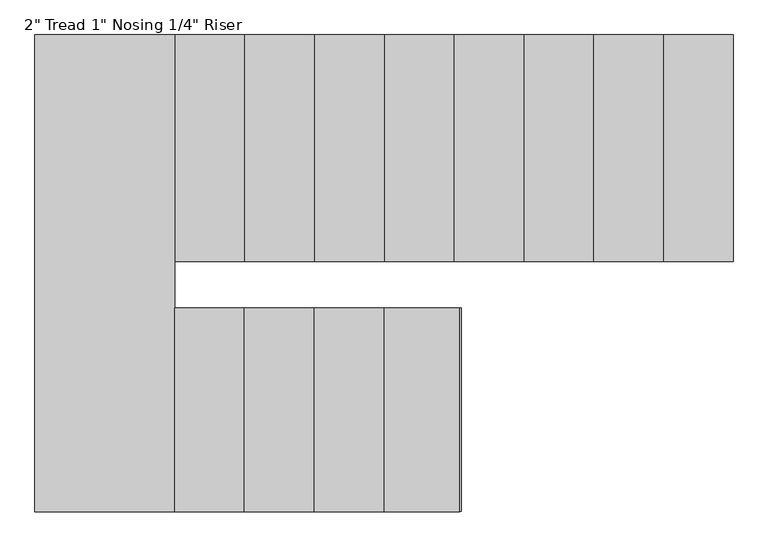
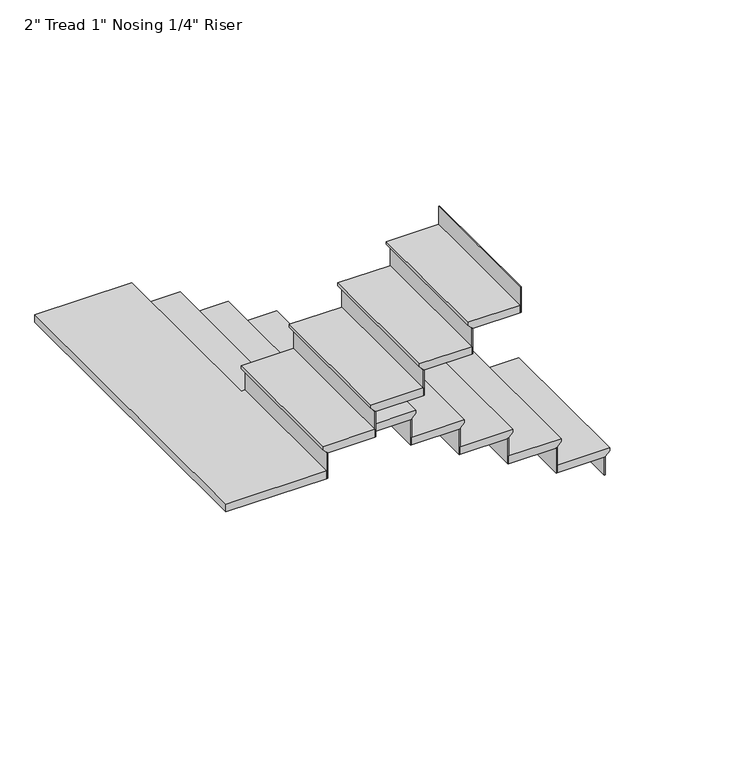
"""IFC4 building model written with IfcOpenShell, lengths in millimetres: stair flight geometry."""

from ifc_helpers import new_model, si_unit, origin, place, context, project, spatial, faceted_brep, source, transform, mapped, element, save


def stair_flight_da212e09(model_context):
    return source(origin(), model_context, "Body", "Brep", [
        faceted_brep([(-569.5630704, 657.3457979, 6398.6833333), (-569.5630704, 657.3457979, 6417.7333333), (-569.5630704, -333.2542021, 6417.7333333), (-569.5630704, -333.2542021, 6398.6833333), (-594.9630704, 657.3457979, 6373.2833333), (-594.9630704, -333.2542021, 6373.2833333), (-899.7630704, 657.3457979, 6417.7333333), (-899.7630704, -333.2542021, 6417.7333333), (-594.9630704, -333.2542021, 6366.9333333), (-899.7630704, -333.2542021, 6366.9333333), (-899.7630704, 657.3457979, 6366.9333333), (-594.9630704, 657.3457979, 6366.9333333)], [[[0, 1, 2, 3]], [[4, 0, 3, 5]], [[2, 1, 6, 7]], [[8, 9, 10, 11]], [[2, 7, 9, 8, 5, 3]], [[8, 11, 4, 5]], [[6, 1, 0, 4, 11, 10]], [[7, 6, 10, 9]]]),
        faceted_brep([(-594.9630704, 657.3457979, 6366.9333333), (-594.9630704, 657.3457979, 6248.4), (-601.3130704, 657.3457979, 6248.4), (-601.3130704, 657.3457979, 6366.9333333), (-594.9630704, -333.2542021, 6366.9333333), (-601.3130704, -333.2542021, 6366.9333333), (-601.3130704, -333.2542021, 6248.4), (-594.9630704, -333.2542021, 6248.4)], [[[0, 1, 2, 3]], [[4, 5, 6, 7]], [[1, 0, 4, 7]], [[2, 1, 7, 6]], [[3, 2, 6, 5]], [[0, 3, 5, 4]]]),
        faceted_brep([(-899.7630704, 657.3457979, 6536.2666667), (-899.7630704, 657.3457979, 6366.9333333), (-906.1130704, 657.3457979, 6366.9333333), (-906.1130704, 657.3457979, 6536.2666667), (-899.7630704, -333.2542021, 6536.2666667), (-906.1130704, -333.2542021, 6536.2666667), (-906.1130704, -333.2542021, 6366.9333333), (-899.7630704, -333.2542021, 6366.9333333)], [[[0, 1, 2, 3]], [[4, 5, 6, 7]], [[1, 0, 4, 7]], [[2, 1, 7, 6]], [[3, 2, 6, 5]], [[0, 3, 5, 4]]]),
        faceted_brep([(-874.3630704, -333.2542021, 6587.0666667), (-874.3630704, 657.3457979, 6587.0666667), (-1204.5630704, 657.3457979, 6587.0666667), (-1204.5630704, -333.2542021, 6587.0666667), (-899.7630704, -333.2542021, 6536.2666667), (-1204.5630704, -333.2542021, 6536.2666667), (-1204.5630704, 657.3457979, 6536.2666667), (-899.7630704, 657.3457979, 6536.2666667), (-899.7630704, -333.2542021, 6542.6166667), (-874.3630704, -333.2542021, 6568.0166667), (-899.7630704, 657.3457979, 6542.6166667), (-874.3630704, 657.3457979, 6568.0166667)], [[[0, 1, 2, 3]], [[4, 5, 6, 7]], [[0, 3, 5, 4, 8, 9]], [[4, 7, 10, 8]], [[2, 1, 11, 10, 7, 6]], [[3, 2, 6, 5]], [[11, 1, 0, 9]], [[10, 11, 9, 8]]]),
        faceted_brep([(-1204.5630704, 657.3457979, 6705.6), (-1204.5630704, 657.3457979, 6536.2666667), (-1210.9130704, 657.3457979, 6536.2666667), (-1210.9130704, 657.3457979, 6705.6), (-1204.5630704, -333.2542021, 6705.6), (-1210.9130704, -333.2542021, 6705.6), (-1210.9130704, -333.2542021, 6536.2666667), (-1204.5630704, -333.2542021, 6536.2666667)], [[[0, 1, 2, 3]], [[4, 5, 6, 7]], [[1, 0, 4, 7]], [[2, 1, 7, 6]], [[3, 2, 6, 5]], [[0, 3, 5, 4]]]),
        faceted_brep([(-1179.1630704, -333.2542021, 6756.4), (-1179.1630704, 657.3457979, 6756.4), (-1509.3630704, 657.3457979, 6756.4), (-1509.3630704, -333.2542021, 6756.4), (-1204.5630704, -333.2542021, 6705.6), (-1509.3630704, -333.2542021, 6705.6), (-1509.3630704, 657.3457979, 6705.6), (-1204.5630704, 657.3457979, 6705.6), (-1204.5630704, -333.2542021, 6711.95), (-1179.1630704, -333.2542021, 6737.35), (-1204.5630704, 657.3457979, 6711.95), (-1179.1630704, 657.3457979, 6737.35)], [[[0, 1, 2, 3]], [[4, 5, 6, 7]], [[0, 3, 5, 4, 8, 9]], [[4, 7, 10, 8]], [[2, 1, 11, 10, 7, 6]], [[3, 2, 6, 5]], [[11, 1, 0, 9]], [[10, 11, 9, 8]]]),
        faceted_brep([(-1509.3630704, 657.3457979, 6874.9333333), (-1509.3630704, 657.3457979, 6705.6), (-1515.7130704, 657.3457979, 6705.6), (-1515.7130704, 657.3457979, 6874.9333333), (-1509.3630704, -333.2542021, 6874.9333333), (-1515.7130704, -333.2542021, 6874.9333333), (-1515.7130704, -333.2542021, 6705.6), (-1509.3630704, -333.2542021, 6705.6)], [[[0, 1, 2, 3]], [[4, 5, 6, 7]], [[1, 0, 4, 7]], [[2, 1, 7, 6]], [[3, 2, 6, 5]], [[0, 3, 5, 4]]]),
        faceted_brep([(-1483.9630704, -333.2542021, 6925.7333333), (-1483.9630704, 657.3457979, 6925.7333333), (-1814.1630704, 657.3457979, 6925.7333333), (-1814.1630704, -333.2542021, 6925.7333333), (-1509.3630704, -333.2542021, 6874.9333333), (-1814.1630704, -333.2542021, 6874.9333333), (-1814.1630704, 657.3457979, 6874.9333333), (-1509.3630704, 657.3457979, 6874.9333333), (-1509.3630704, -333.2542021, 6881.2833333), (-1483.9630704, -333.2542021, 6906.6833333), (-1509.3630704, 657.3457979, 6881.2833333), (-1483.9630704, 657.3457979, 6906.6833333)], [[[0, 1, 2, 3]], [[4, 5, 6, 7]], [[0, 3, 5, 4, 8, 9]], [[4, 7, 10, 8]], [[2, 1, 11, 10, 7, 6]], [[3, 2, 6, 5]], [[11, 1, 0, 9]], [[10, 11, 9, 8]]]),
        faceted_brep([(-1814.1630704, 657.3457979, 7044.2666667), (-1814.1630704, 657.3457979, 6874.9333333), (-1820.5130704, 657.3457979, 6874.9333333), (-1820.5130704, 657.3457979, 7044.2666667), (-1814.1630704, -333.2542021, 7044.2666667), (-1820.5130704, -333.2542021, 7044.2666667), (-1820.5130704, -333.2542021, 6874.9333333), (-1814.1630704, -333.2542021, 6874.9333333)], [[[0, 1, 2, 3]], [[4, 5, 6, 7]], [[1, 0, 4, 7]], [[2, 1, 7, 6]], [[3, 2, 6, 5]], [[0, 3, 5, 4]]]),
        faceted_brep([(-1788.7630704, -333.2542021, 7095.0666667), (-1788.7630704, 657.3457979, 7095.0666667), (-2118.9630704, 657.3457979, 7095.0666667), (-2118.9630704, -333.2542021, 7095.0666667), (-1814.1630704, -333.2542021, 7044.2666667), (-2118.9630704, -333.2542021, 7044.2666667), (-2118.9630704, 657.3457979, 7044.2666667), (-1814.1630704, 657.3457979, 7044.2666667), (-1814.1630704, -333.2542021, 7050.6166667), (-1788.7630704, -333.2542021, 7076.0166667), (-1814.1630704, 657.3457979, 7050.6166667), (-1788.7630704, 657.3457979, 7076.0166667)], [[[0, 1, 2, 3]], [[4, 5, 6, 7]], [[0, 3, 5, 4, 8, 9]], [[4, 7, 10, 8]], [[2, 1, 11, 10, 7, 6]], [[3, 2, 6, 5]], [[11, 1, 0, 9]], [[10, 11, 9, 8]]]),
        faceted_brep([(-2118.9630704, 657.3457979, 7213.6), (-2118.9630704, 657.3457979, 7044.2666667), (-2125.3130704, 657.3457979, 7044.2666667), (-2125.3130704, 657.3457979, 7213.6), (-2118.9630704, -333.2542021, 7213.6), (-2125.3130704, -333.2542021, 7213.6), (-2125.3130704, -333.2542021, 7044.2666667), (-2118.9630704, -333.2542021, 7044.2666667)], [[[0, 1, 2, 3]], [[4, 5, 6, 7]], [[1, 0, 4, 7]], [[2, 1, 7, 6]], [[3, 2, 6, 5]], [[0, 3, 5, 4]]]),
        faceted_brep([(-2093.5630704, -333.2542021, 7264.4), (-2093.5630704, 657.3457979, 7264.4), (-2423.7630704, 657.3457979, 7264.4), (-2423.7630704, -333.2542021, 7264.4), (-2118.9630704, -333.2542021, 7213.6), (-2423.7630704, -333.2542021, 7213.6), (-2423.7630704, 657.3457979, 7213.6), (-2118.9630704, 657.3457979, 7213.6), (-2118.9630704, -333.2542021, 7219.95), (-2093.5630704, -333.2542021, 7245.35), (-2118.9630704, 657.3457979, 7219.95), (-2093.5630704, 657.3457979, 7245.35)], [[[0, 1, 2, 3]], [[4, 5, 6, 7]], [[0, 3, 5, 4, 8, 9]], [[4, 7, 10, 8]], [[2, 1, 11, 10, 7, 6]], [[3, 2, 6, 5]], [[11, 1, 0, 9]], [[10, 11, 9, 8]]]),
        faceted_brep([(-2423.7630704, 657.3457979, 7382.9333333), (-2423.7630704, 657.3457979, 7213.6), (-2430.1130704, 657.3457979, 7213.6), (-2430.1130704, 657.3457979, 7382.9333333), (-2423.7630704, -333.2542021, 7382.9333333), (-2430.1130704, -333.2542021, 7382.9333333), (-2430.1130704, -333.2542021, 7213.6), (-2423.7630704, -333.2542021, 7213.6)], [[[0, 1, 2, 3]], [[4, 5, 6, 7]], [[1, 0, 4, 7]], [[2, 1, 7, 6]], [[3, 2, 6, 5]], [[0, 3, 5, 4]]]),
        faceted_brep([(-2398.3630704, -333.2542021, 7433.7333333), (-2398.3630704, 657.3457979, 7433.7333333), (-2728.5630704, 657.3457979, 7433.7333333), (-2728.5630704, -333.2542021, 7433.7333333), (-2423.7630704, -333.2542021, 7382.9333333), (-2728.5630704, -333.2542021, 7382.9333333), (-2728.5630704, 657.3457979, 7382.9333333), (-2423.7630704, 657.3457979, 7382.9333333), (-2423.7630704, -333.2542021, 7389.2833333), (-2398.3630704, -333.2542021, 7414.6833333), (-2423.7630704, 657.3457979, 7389.2833333), (-2398.3630704, 657.3457979, 7414.6833333)], [[[0, 1, 2, 3]], [[4, 5, 6, 7]], [[0, 3, 5, 4, 8, 9]], [[4, 7, 10, 8]], [[2, 1, 11, 10, 7, 6]], [[3, 2, 6, 5]], [[11, 1, 0, 9]], [[10, 11, 9, 8]]]),
        faceted_brep([(-2728.5630704, 657.3457979, 7552.2666667), (-2728.5630704, 657.3457979, 7382.9333333), (-2734.9130704, 657.3457979, 7382.9333333), (-2734.9130704, 657.3457979, 7552.2666667), (-2728.5630704, -333.2542021, 7552.2666667), (-2734.9130704, -333.2542021, 7552.2666667), (-2734.9130704, -333.2542021, 7382.9333333), (-2728.5630704, -333.2542021, 7382.9333333)], [[[0, 1, 2, 3]], [[4, 5, 6, 7]], [[1, 0, 4, 7]], [[2, 1, 7, 6]], [[3, 2, 6, 5]], [[0, 3, 5, 4]]]),
        faceted_brep([(-2703.1630704, -333.2542021, 7603.0666667), (-2703.1630704, 657.3457979, 7603.0666667), (-3033.3630704, 657.3457979, 7603.0666667), (-3033.3630704, -333.2542021, 7603.0666667), (-2728.5630704, -333.2542021, 7552.2666667), (-3033.3630704, -333.2542021, 7552.2666667), (-3033.3630704, 657.3457979, 7552.2666667), (-2728.5630704, 657.3457979, 7552.2666667), (-2728.5630704, -333.2542021, 7558.6166667), (-2703.1630704, -333.2542021, 7584.0166667), (-2728.5630704, 657.3457979, 7558.6166667), (-2703.1630704, 657.3457979, 7584.0166667)], [[[0, 1, 2, 3]], [[4, 5, 6, 7]], [[0, 3, 5, 4, 8, 9]], [[4, 7, 10, 8]], [[2, 1, 11, 10, 7, 6]], [[3, 2, 6, 5]], [[11, 1, 0, 9]], [[10, 11, 9, 8]]]),
        faceted_brep([(-3033.3630704, 657.3457979, 7721.6), (-3033.3630704, 657.3457979, 7552.2666667), (-3039.7130704, 657.3457979, 7552.2666667), (-3039.7130704, 657.3457979, 7721.6), (-3033.3630704, -333.2542021, 7721.6), (-3039.7130704, -333.2542021, 7721.6), (-3039.7130704, -333.2542021, 7552.2666667), (-3033.3630704, -333.2542021, 7552.2666667)], [[[0, 1, 2, 3]], [[4, 5, 6, 7]], [[1, 0, 4, 7]], [[2, 1, 7, 6]], [[3, 2, 6, 5]], [[0, 3, 5, 4]]]),
        faceted_brep([(-2982.5630704, -536.4542021, 7772.4), (-3007.9630704, -536.4542021, 7772.4), (-3007.9630704, 657.3457979, 7772.4), (-3617.5630704, 657.3457979, 7772.4), (-3617.5630704, -1425.4542021, 7772.4), (-2982.5630704, -1425.4542021, 7772.4), (-3007.9630704, -536.4542021, 7721.6), (-2982.5630704, -536.4542021, 7721.6), (-2982.5630704, -1425.4542021, 7721.6), (-3617.5630704, -1425.4542021, 7721.6), (-3617.5630704, 657.3457979, 7721.6), (-3033.3630704, 657.3457979, 7721.6), (-3033.3630704, -333.2542021, 7721.6), (-3007.9630704, -333.2542021, 7721.6), (-3007.9630704, -333.2542021, 7753.35), (-3007.9630704, 657.3457979, 7753.35), (-3033.3630704, -333.2542021, 7727.95), (-3033.3630704, 657.3457979, 7727.95)], [[[0, 1, 2, 3, 4, 5]], [[6, 7, 8, 9, 10, 11, 12, 13]], [[1, 0, 7, 6]], [[2, 1, 6, 13, 14, 15]], [[13, 12, 16, 14]], [[12, 11, 17, 16]], [[3, 2, 15, 17, 11, 10]], [[4, 3, 10, 9]], [[5, 4, 9, 8]], [[0, 5, 8, 7]], [[17, 15, 14, 16]]]),
        faceted_brep([(-2982.5630704, -1425.4542021, 7890.9333333), (-2982.5630704, -1425.4542021, 7721.6), (-2976.2130704, -1425.4542021, 7721.6), (-2976.2130704, -1425.4542021, 7890.9333333), (-2982.5630704, -536.4542021, 7890.9333333), (-2976.2130704, -536.4542021, 7890.9333333), (-2976.2130704, -536.4542021, 7721.6), (-2982.5630704, -536.4542021, 7721.6)], [[[0, 1, 2, 3]], [[4, 5, 6, 7]], [[1, 0, 4, 7]], [[2, 1, 7, 6]], [[3, 2, 6, 5]], [[0, 3, 5, 4]]]),
        faceted_brep([(-3007.9630704, -536.4542021, 7941.7333333), (-3007.9630704, -1425.4542021, 7941.7333333), (-2677.7630704, -1425.4542021, 7941.7333333), (-2677.7630704, -536.4542021, 7941.7333333), (-2982.5630704, -536.4542021, 7890.9333333), (-2677.7630704, -536.4542021, 7890.9333333), (-2677.7630704, -1425.4542021, 7890.9333333), (-2982.5630704, -1425.4542021, 7890.9333333), (-2982.5630704, -536.4542021, 7897.2833333), (-3007.9630704, -536.4542021, 7922.6833333), (-2982.5630704, -1425.4542021, 7897.2833333), (-3007.9630704, -1425.4542021, 7922.6833333)], [[[0, 1, 2, 3]], [[4, 5, 6, 7]], [[0, 3, 5, 4, 8, 9]], [[4, 7, 10, 8]], [[2, 1, 11, 10, 7, 6]], [[3, 2, 6, 5]], [[11, 1, 0, 9]], [[10, 11, 9, 8]]]),
        faceted_brep([(-2677.7630704, -1425.4542021, 8060.2666667), (-2677.7630704, -1425.4542021, 7890.9333333), (-2671.4130704, -1425.4542021, 7890.9333333), (-2671.4130704, -1425.4542021, 8060.2666667), (-2677.7630704, -536.4542021, 8060.2666667), (-2671.4130704, -536.4542021, 8060.2666667), (-2671.4130704, -536.4542021, 7890.9333333), (-2677.7630704, -536.4542021, 7890.9333333)], [[[0, 1, 2, 3]], [[4, 5, 6, 7]], [[1, 0, 4, 7]], [[2, 1, 7, 6]], [[3, 2, 6, 5]], [[0, 3, 5, 4]]]),
        faceted_brep([(-2703.1630704, -536.4542021, 8111.0666667), (-2703.1630704, -1425.4542021, 8111.0666667), (-2372.9630704, -1425.4542021, 8111.0666667), (-2372.9630704, -536.4542021, 8111.0666667), (-2677.7630704, -536.4542021, 8060.2666667), (-2372.9630704, -536.4542021, 8060.2666667), (-2372.9630704, -1425.4542021, 8060.2666667), (-2677.7630704, -1425.4542021, 8060.2666667), (-2677.7630704, -536.4542021, 8066.6166667), (-2703.1630704, -536.4542021, 8092.0166667), (-2677.7630704, -1425.4542021, 8066.6166667), (-2703.1630704, -1425.4542021, 8092.0166667)], [[[0, 1, 2, 3]], [[4, 5, 6, 7]], [[0, 3, 5, 4, 8, 9]], [[4, 7, 10, 8]], [[2, 1, 11, 10, 7, 6]], [[3, 2, 6, 5]], [[11, 1, 0, 9]], [[10, 11, 9, 8]]]),
        faceted_brep([(-2372.9630704, -1425.4542021, 8229.6), (-2372.9630704, -1425.4542021, 8060.2666667), (-2366.6130704, -1425.4542021, 8060.2666667), (-2366.6130704, -1425.4542021, 8229.6), (-2372.9630704, -536.4542021, 8229.6), (-2366.6130704, -536.4542021, 8229.6), (-2366.6130704, -536.4542021, 8060.2666667), (-2372.9630704, -536.4542021, 8060.2666667)], [[[0, 1, 2, 3]], [[4, 5, 6, 7]], [[1, 0, 4, 7]], [[2, 1, 7, 6]], [[3, 2, 6, 5]], [[0, 3, 5, 4]]]),
        faceted_brep([(-2398.3630704, -536.4542021, 8280.4), (-2398.3630704, -1425.4542021, 8280.4), (-2068.1630704, -1425.4542021, 8280.4), (-2068.1630704, -536.4542021, 8280.4), (-2372.9630704, -536.4542021, 8229.6), (-2068.1630704, -536.4542021, 8229.6), (-2068.1630704, -1425.4542021, 8229.6), (-2372.9630704, -1425.4542021, 8229.6), (-2372.9630704, -536.4542021, 8235.95), (-2398.3630704, -536.4542021, 8261.35), (-2372.9630704, -1425.4542021, 8235.95), (-2398.3630704, -1425.4542021, 8261.35)], [[[0, 1, 2, 3]], [[4, 5, 6, 7]], [[0, 3, 5, 4, 8, 9]], [[4, 7, 10, 8]], [[2, 1, 11, 10, 7, 6]], [[3, 2, 6, 5]], [[11, 1, 0, 9]], [[10, 11, 9, 8]]]),
        faceted_brep([(-2068.1630704, -1425.4542021, 8398.9333333), (-2068.1630704, -1425.4542021, 8229.6), (-2061.8130704, -1425.4542021, 8229.6), (-2061.8130704, -1425.4542021, 8398.9333333), (-2068.1630704, -536.4542021, 8398.9333333), (-2061.8130704, -536.4542021, 8398.9333333), (-2061.8130704, -536.4542021, 8229.6), (-2068.1630704, -536.4542021, 8229.6)], [[[0, 1, 2, 3]], [[4, 5, 6, 7]], [[1, 0, 4, 7]], [[2, 1, 7, 6]], [[3, 2, 6, 5]], [[0, 3, 5, 4]]]),
        faceted_brep([(-1763.3630704, -1425.4542021, 8568.2666667), (-1763.3630704, -1425.4542021, 8398.9333333), (-1757.0130704, -1425.4542021, 8398.9333333), (-1757.0130704, -1425.4542021, 8568.2666667), (-1763.3630704, -536.4542021, 8568.2666667), (-1757.0130704, -536.4542021, 8568.2666667), (-1757.0130704, -536.4542021, 8398.9333333), (-1763.3630704, -536.4542021, 8398.9333333)], [[[0, 1, 2, 3]], [[4, 5, 6, 7]], [[1, 0, 4, 7]], [[2, 1, 7, 6]], [[3, 2, 6, 5]], [[0, 3, 5, 4]]]),
        faceted_brep([(-2093.5630704, -536.4542021, 8449.7333333), (-2093.5630704, -1425.4542021, 8449.7333333), (-1763.3630704, -1425.4542021, 8449.7333333), (-1763.3630704, -536.4542021, 8449.7333333), (-2068.1630704, -536.4542021, 8398.9333333), (-1763.3630704, -536.4542021, 8398.9333333), (-1763.3630704, -1425.4542021, 8398.9333333), (-2068.1630704, -1425.4542021, 8398.9333333), (-2068.1630704, -536.4542021, 8405.2833333), (-2093.5630704, -536.4542021, 8430.6833333), (-2068.1630704, -1425.4542021, 8405.2833333), (-2093.5630704, -1425.4542021, 8430.6833333)], [[[0, 1, 2, 3]], [[4, 5, 6, 7]], [[0, 3, 5, 4, 8, 9]], [[4, 7, 10, 8]], [[2, 1, 11, 10, 7, 6]], [[3, 2, 6, 5]], [[11, 1, 0, 9]], [[10, 11, 9, 8]]]),
    ])


if __name__ == "__main__":
    model = new_model("IFC4")
    model_context = context("Model", 3, world=origin())
    ifc_project = project(units=[si_unit("LENGTHUNIT", "METRE", prefix="MILLI")], contexts=[model_context])
    site = spatial("IfcSite", under=ifc_project)
    building = spatial("IfcBuilding", under=site)
    placement = place(None, origin())
    stair_flight_shape = stair_flight_da212e09(model_context)
    element("IfcStairFlight", 1, ObjectType="2\" Tread 1\" Nosing 1/4\" Riser", at=placement, inside=building, context=model_context, shape_type="MappedRepresentation", body=[
        mapped(stair_flight_shape, transform((0.0, 0.0, 0.0), x_axis=(1.0, 0.0, 0.0), y_axis=(0.0, 1.0, 0.0), z_axis=(0.0, 0.0, 1.0))),
    ])
    save(model, "model.ifc")
